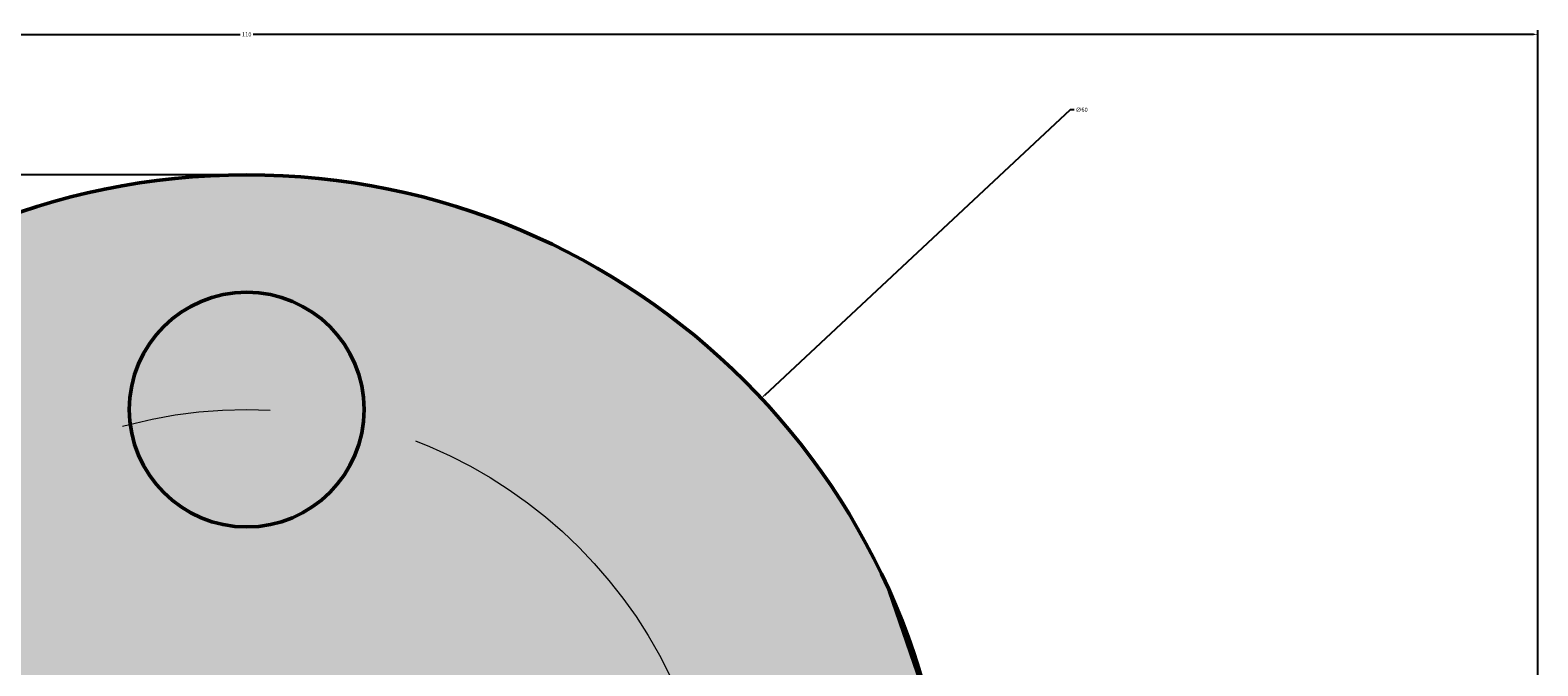
# Model space of a CAD drawing. Units: inches. Extents: x 114 to 236, y -51 to 115.
# Tile 14 of 14: x 166 to 230, y 88 to 115. Entities that reach past the tile are written whole.
import ezdxf

# ---------------------------------------------------------------- set-up
doc = ezdxf.new("R2010")
doc.units = ezdxf.units.IN
doc.header["$MEASUREMENT"] = 0
doc.linetypes.add('CENTER', pattern=[50.8, 31.75, -6.35, 6.35, -6.35])
for name, color, linetype, lineweight in [('M-CNTR', 7, 'CENTER', 18), ('M-DIMS', 2, 'Continuous', 18), ('M-OUTL', 7, 'Continuous', 50)]:
    doc.layers.add(name, color=color, linetype=linetype, lineweight=lineweight)
doc.layers.add('M-HATC', color=7, linetype='Continuous', lineweight=18, true_color=0xffffff)
doc.styles.get("Standard").update_dxf_attribs({"font": 'arial.ttf'})
doc.dimstyles.get("Standard").update_dxf_attribs({"dimtxt": 0.18, "dimasz": 0.18, "dimexe": 0.18, "dimexo": 0.0625, "dimgap": 0.09, "dimtad": 0, "dimtih": 1, "dimtoh": 1, "dimdec": 4, "dimzin": 0, "dimdsep": 46, "dimtxsty": 'Standard', "dimcen": 0.09, "dimadec": 0, "dimazin": 0, "dimtfac": 1, "dimtdec": 4, "dimtofl": 0, "dimtmove": 0, "dimatfit": 3, "dimfxl": 1, "dimtolj": 1, "dimtzin": 0, "dimarcsym": 0})

# ---------------------------------------------------------------- blocks, each defined once
blk = doc.blocks.new('BOLT-HOLE-D10')
blk.add_circle((0, 0), 5)
blk = doc.blocks.new('*D3')
at = {"layer": 'Defpoints', "color": 0, "transparency": 16777216}
for p in [(230.229, 115.287), (120.229, 9.307), (230.229, 9.307)]:
    blk.add_point(p, dxfattribs=at)
at = {"layer": 'M-DIMS', "color": 0, "lineweight": -2, "transparency": 16777216}
for p, q in [((120.229, 9.37), (120.229, 115.467)), ((120.409, 115.287), (174.949, 115.287)), ((230.049, 115.287), (175.509, 115.287)), ((230.229, 9.37), (230.229, 115.467))]:
    blk.add_line(p, q, dxfattribs=at)
at = {"layer": 'M-DIMS', "color": 0, "transparency": 16777216}
for points in [[(120.409, 115.317), (120.409, 115.257), (120.229, 115.287)], [(230.049, 115.317), (230.049, 115.257), (230.229, 115.287)]]:
    blk.add_solid(points, dxfattribs=at)
at = {"layer": 'M-DIMS', "color": 0, "transparency": 16777216, "insert": (175.229, 115.287), "char_height": 0.18, "attachment_point": 5}
blk.add_mtext('\\A1;110', dxfattribs=at)
blk = doc.blocks.new('*D4')
at = {"layer": 'Defpoints', "color": 0, "transparency": 16777216}
for p in [(114.249, 109.307), (175.229, 109.307), (135.229, -5.693)]:
    blk.add_point(p, dxfattribs=at)
at = {"layer": 'M-DIMS', "color": 0, "lineweight": -2, "transparency": 16777216}
for p, q in [((175.166, 109.307), (114.069, 109.307)), ((114.249, 109.127), (114.249, 51.989)), ((114.249, -5.513), (114.249, 51.625)), ((135.166, -5.693), (114.069, -5.693))]:
    blk.add_line(p, q, dxfattribs=at)
at = {"layer": 'M-DIMS', "color": 0, "transparency": 16777216}
for points in [[(114.219, 109.127), (114.279, 109.127), (114.249, 109.307)], [(114.219, -5.513), (114.279, -5.513), (114.249, -5.693)]]:
    blk.add_solid(points, dxfattribs=at)
at = {"layer": 'M-DIMS', "color": 0, "transparency": 16777216, "insert": (114.249, 51.807), "char_height": 0.18, "attachment_point": 5}
blk.add_mtext('\\A1;115', dxfattribs=at)
blk = doc.blocks.new('*D8')
at = {"layer": 'Defpoints', "color": 0, "transparency": 16777216}
for p in [(197.149, 99.789), (153.308, 58.825)]:
    blk.add_point(p, dxfattribs=at)
at = {"layer": 'M-DIMS', "color": 0, "lineweight": -2, "transparency": 16777216}
for p, q in [((210.301, 112.078), (197.28, 99.912)), ((210.481, 112.078), (210.301, 112.078)), ((175.139, 79.307), (175.319, 79.307)), ((175.229, 79.217), (175.229, 79.397))]:
    blk.add_line(p, q, dxfattribs=at)
at = {"layer": 'M-DIMS', "color": 0, "transparency": 16777216}
blk.add_solid([(197.26, 99.934), (197.301, 99.89), (197.149, 99.789)], dxfattribs=at)
at = {"layer": 'M-DIMS', "color": 0, "transparency": 16777216, "insert": (210.797, 112.078), "char_height": 0.18, "attachment_point": 5}
blk.add_mtext('\\A1;∅60', dxfattribs=at)
blk = doc.blocks.new('*D9')
at = {"layer": 'Defpoints', "color": 0, "transparency": 16777216}
for p in [(157.908, 89.307), (192.549, 69.307)]:
    blk.add_point(p, dxfattribs=at)
at = {"layer": 'M-DIMS', "color": 0, "lineweight": -2, "transparency": 16777216}
for p, q in [((147.336, 95.307), (147.516, 95.307)), ((147.516, 95.307), (157.752, 89.397)), ((175.139, 79.307), (175.319, 79.307)), ((175.229, 79.217), (175.229, 79.397))]:
    blk.add_line(p, q, dxfattribs=at)
at = {"layer": 'M-DIMS', "color": 0, "transparency": 16777216}
blk.add_solid([(157.767, 89.423), (157.737, 89.371), (157.908, 89.307)], dxfattribs=at)
at = {"layer": 'M-DIMS', "color": 0, "transparency": 16777216, "insert": (147.019, 95.307), "char_height": 0.18, "attachment_point": 5}
blk.add_mtext('\\A1;∅40', dxfattribs=at)

msp = doc.modelspace()

# ---------------------------------------------------------------- hatches: boundary and pattern name
at = {"layer": 'M-HATC'}
h = msp.add_hatch(color=256, dxfattribs=at)
h.set_gradient(color1=(19, 155, 72), color2=(255, 255, 0), tint=1, name='HEMISPHERICAL')
h.paths.add_polyline_path([(147.853, 91.577), (146.105, 86.505, 0.060651), (145.229, 79.307, 1), (205.229, 79.307, 0.060651), (204.352, 86.505), (202.605, 91.577, 0.647643)])
h.paths.add_polyline_path([(180.229, 99.307, -0.031342), (180.189, 98.682, -0.27393), (194.604, 84.268, -0.451416), (200.229, 79.307, -0.451416), (194.604, 74.346, -0.27393), (180.189, 59.932, -0.031342), (180.229, 59.307, -1), (170.229, 59.307, -0.031342), (170.268, 59.932, -0.27393), (155.854, 74.346, -0.451416), (150.229, 79.307, -0.451416), (155.854, 84.268, -0.27393), (170.268, 98.682, -0.031342), (170.229, 99.307, -1)], flags=16)
h.paths.add_polyline_path([(183.229, 79.307, -1), (167.229, 79.307, -1)], flags=0)
h.paths.add_polyline_path([(155.854, 84.268, -0.377964), (160.229, 79.307, -0.377964), (155.854, 74.346, 0.27393), (170.268, 59.932, -0.881917), (180.189, 59.932, 0.27393), (194.604, 74.346, -0.377964), (190.229, 79.307, -0.377964), (194.604, 84.268, 0.27393), (180.189, 98.682, -0.881917), (170.268, 98.682, 0.27393)], flags=0)
h = msp.add_hatch(color=256, dxfattribs=at)
h.paths.add_polyline_path([(170.268, 98.682, 0.881917), (180.189, 98.682, 0.125988)])
h.paths.add_polyline_path([(170.229, 99.307, 0.031342), (170.268, 98.682, -0.125988), (180.189, 98.682, 0.031342), (180.229, 99.307, 1)])

# ---------------------------------------------------------------- linework, layer by layer
at = {"layer": 'M-CNTR'}
msp.add_circle((175.229, 79.307), 20, dxfattribs=at)
at = {"layer": 'M-OUTL'}
msp.add_line((229.935, 12.263), (202.605, 91.577), dxfattribs=at)
msp.add_circle((175.229, 79.307), 30, dxfattribs=at)

# ---------------------------------------------------------------- block references
msp.add_blockref('BOLT-HOLE-D10', (175.229, 99.307), dxfattribs=at)

# ---------------------------------------------------------------- dimensions: what is measured, and where the dimension line sits
at = {"layer": 'M-DIMS'}
dim = msp.add_linear_dim(base=(230.229, 115.287), p1=(120.229, 9.307), p2=(230.229, 9.307), dimstyle='Standard', override={"dimdec": 0, "dimlfac": 1, "dimrnd": 0, "dimzin": 0, "dimdsep": 46, "dimlunit": 2}, dxfattribs=at)
dim.commit()
dim.dimension.update_dxf_attribs({"geometry": '*D3', "text_midpoint": (175.229, 115.287)})
for p1, p2, picture, middle in [((153.308, 58.825), (197.149, 99.789), '*D8', (210.797, 112.078)), ((192.549, 69.307), (157.908, 89.307), '*D9', (147.019, 95.307))]:
    dim = msp.add_diameter_dim_2p(p1=p1, p2=p2, dimstyle='Standard', override={"dimdec": 0, "dimlfac": 1, "dimrnd": 0, "dimzin": 0, "dimdsep": 46, "dimlunit": 2}, dxfattribs=at)
    dim.commit()
    dim.dimension.update_dxf_attribs({"geometry": picture, "text_midpoint": middle, "dimtype": 163})
dim = msp.add_linear_dim(base=(114.249, 109.307), p1=(135.229, -5.693), p2=(175.229, 109.307), angle=90, dimstyle='Standard', override={"dimdec": 0, "dimlfac": 1, "dimrnd": 0, "dimzin": 0, "dimdsep": 46, "dimlunit": 2}, dxfattribs=at)
dim.commit()
dim.dimension.update_dxf_attribs({"geometry": '*D4', "text_midpoint": (114.249, 51.807)})

doc.saveas('drawing.dxf')
